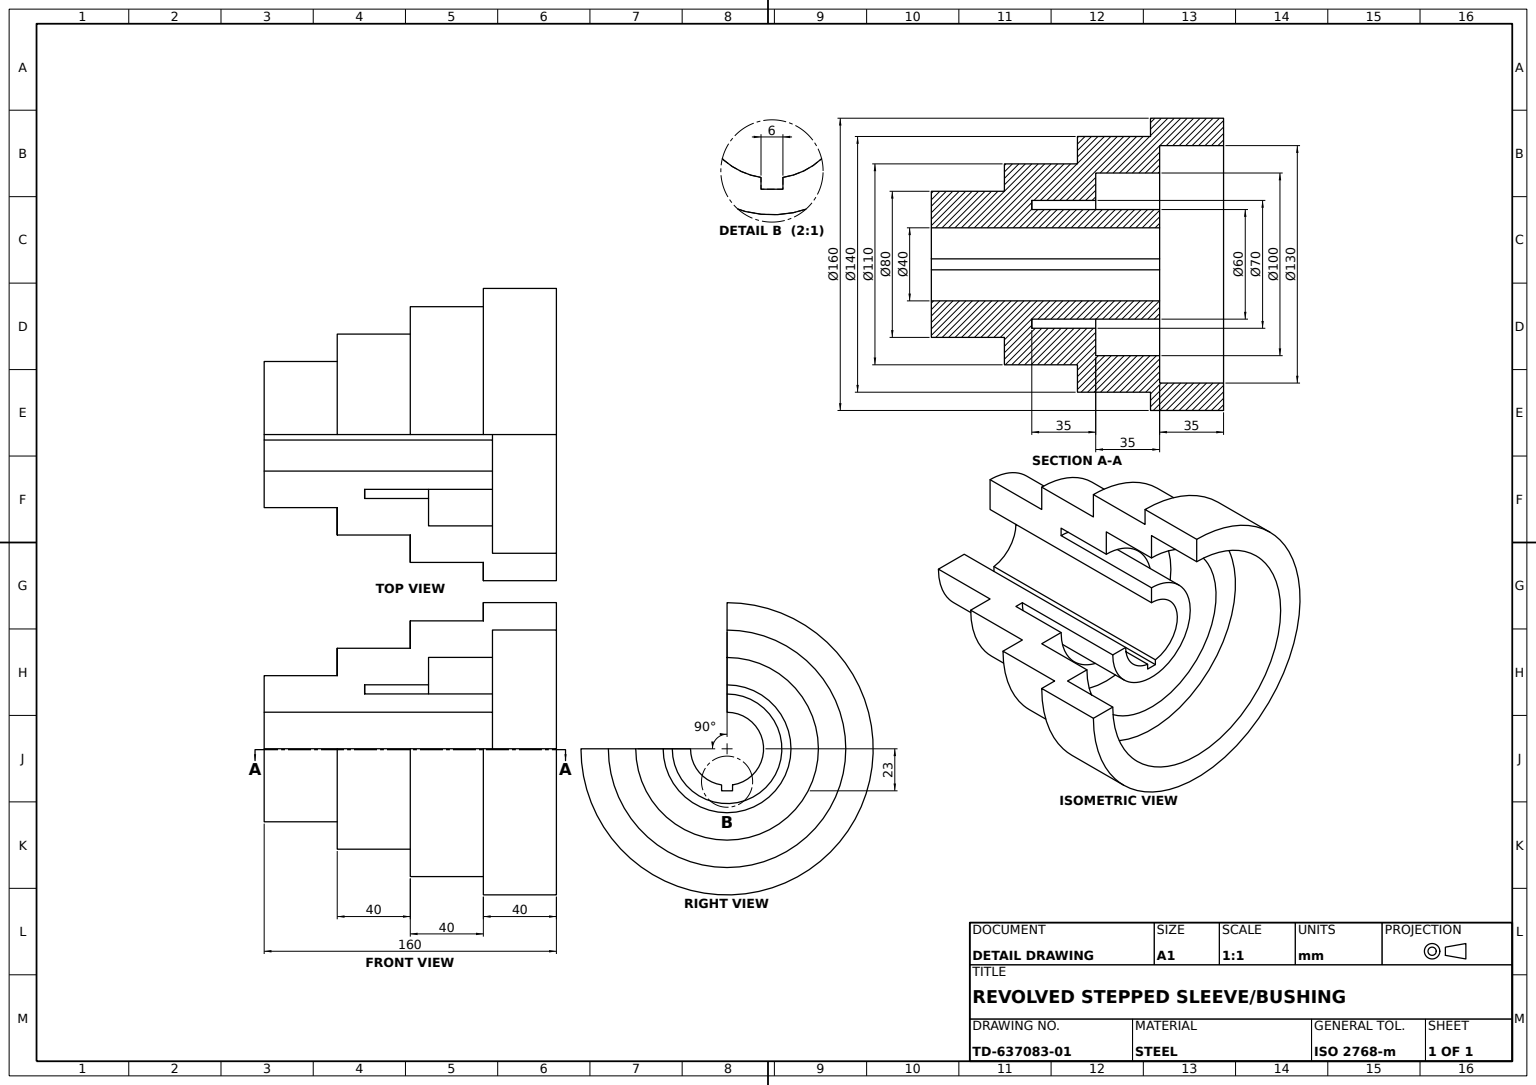
from build123d import *

# Parameters (mm, degrees)
STEPPED_PULLEY_BODY_ANGLE  = 270
KEYWAY_SLOT_6X3_DEPTH      = 196.959179423
KEYWAY_SLOT_6X3_DEPTH_BACK = 196.959179423


with BuildPart() as part:
    # Pulley Profile Sketch → Stepped Pulley Body (revolve)
    with BuildSketch(Plane.XY):
        Polygon((0, 40), (0, 20), (125, 20), (125, 30), (55, 30), (55, 35), (90, 35), (90, 50), (125, 50), (125, 65), (160, 65), (160, 80), (120, 80), (120, 70), (80, 70), (80, 55), (40, 55), (40, 40), align=None)
    revolve(axis=Axis((125, 0, 0), (-1, 0, 0)), revolution_arc=STEPPED_PULLEY_BODY_ANGLE)

    # Keyway Slot Sketch → Keyway Slot 6x3 (cut, two sides: drawn at the far end of the back side and taken through both)
    with BuildSketch(Plane(origin=(0, 0, 0), x_dir=(0, 0, -1), z_dir=(1, 0, 0)).offset(-KEYWAY_SLOT_6X3_DEPTH_BACK)):
        with BuildLine():
            ThreePointArc((3, -19.773719933), (1.504260837, -19.943349752), (0, -20))
            Line((0, -20), (0, -23))
            Line((0, -23), (3, -23))
            Line((3, -23), (3, -19.773719933))
        make_face()
        with BuildLine():
            Line((0, -23), (0, -20))
            ThreePointArc((0, -20), (-1.504260837, -19.943349752), (-3, -19.773719933))
            Line((-3, -19.773719933), (-3, -23))
            Line((-3, -23), (0, -23))
        make_face()
    extrude(amount=KEYWAY_SLOT_6X3_DEPTH + KEYWAY_SLOT_6X3_DEPTH_BACK, mode=Mode.SUBTRACT)


solid = part.part
